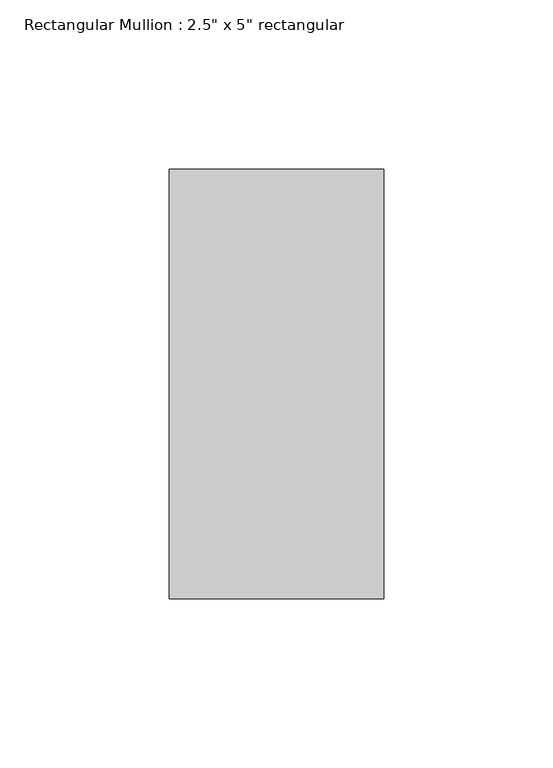
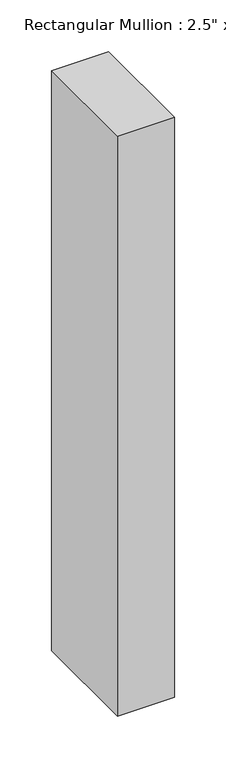
"""IFC4 building model written with IfcOpenShell, lengths in millimetres: member geometry."""

from ifc_helpers import new_model, si_unit, frame, origin, place, context, project, spatial, polyline, outline, extrude, source, transform, mapped, element, save


def member_187b6476(model_context):
    return source(origin(), model_context, "Body", "SweptSolid", [
        extrude(outline(polyline([(0.0, 63.5), (0.0, -63.5), (-63.5, -63.5), (-63.5, 63.5), (0.0, 63.5)])), frame((0.0, 0.0, -683.7625925), z_axis=(0.0, 0.0, 1.0), x_axis=(1.0, 0.0, 0.0)), (0.0, 0.0, 1.0), 683.7625925),
    ])


if __name__ == "__main__":
    model = new_model("IFC4")
    model_context = context("Model", 3, world=origin())
    ifc_project = project(units=[si_unit("LENGTHUNIT", "METRE", prefix="MILLI")], contexts=[model_context])
    site = spatial("IfcSite", under=ifc_project)
    building = spatial("IfcBuilding", under=site)
    placement = place(None, origin())
    member_shape = member_187b6476(model_context)
    element("IfcMember", 1, ObjectType="Rectangular Mullion : 2.5\" x 5\" rectangular", at=placement, inside=building, context=model_context, shape_type="MappedRepresentation", body=[
        mapped(member_shape, transform((0.0, 0.0, 0.0), x_axis=(1.0, 0.0, 0.0), y_axis=(0.0, 1.0, 0.0), z_axis=(0.0, 0.0, 1.0))),
    ])
    save(model, "model.ifc")

# Revit data of these elements
# Type "Rectangular Mullion : 2.5\" x 5\" rectangular"
#   built-in parameter 1007304 = 0.416667 (stored number, unit not read)
#   built-in parameter 1007301 = 0.104167 (stored number, unit not read)
#   built-in parameter 1007300 = 0.104167 (stored number, unit not read)
# Element 1 (IfcMember, "Rectangular Mullion : 2.5\" x 5\" rectangular")
#   Materials on its faces: "Aluminum"
# Materials
#   "Aluminum": class "Metal", colour RGB 247 247 247, transparency 0, Description = "Aluminum 6061", Cost = 0
